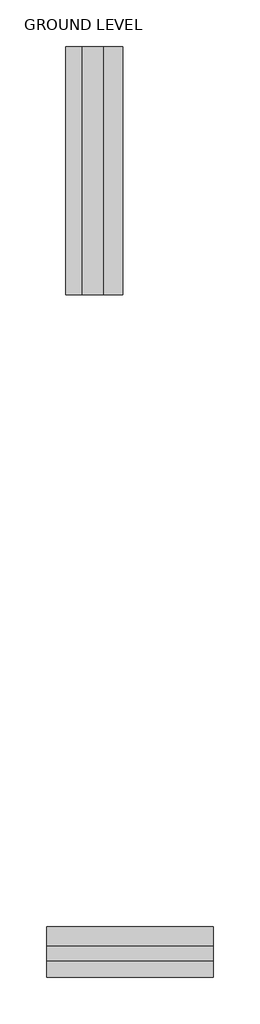
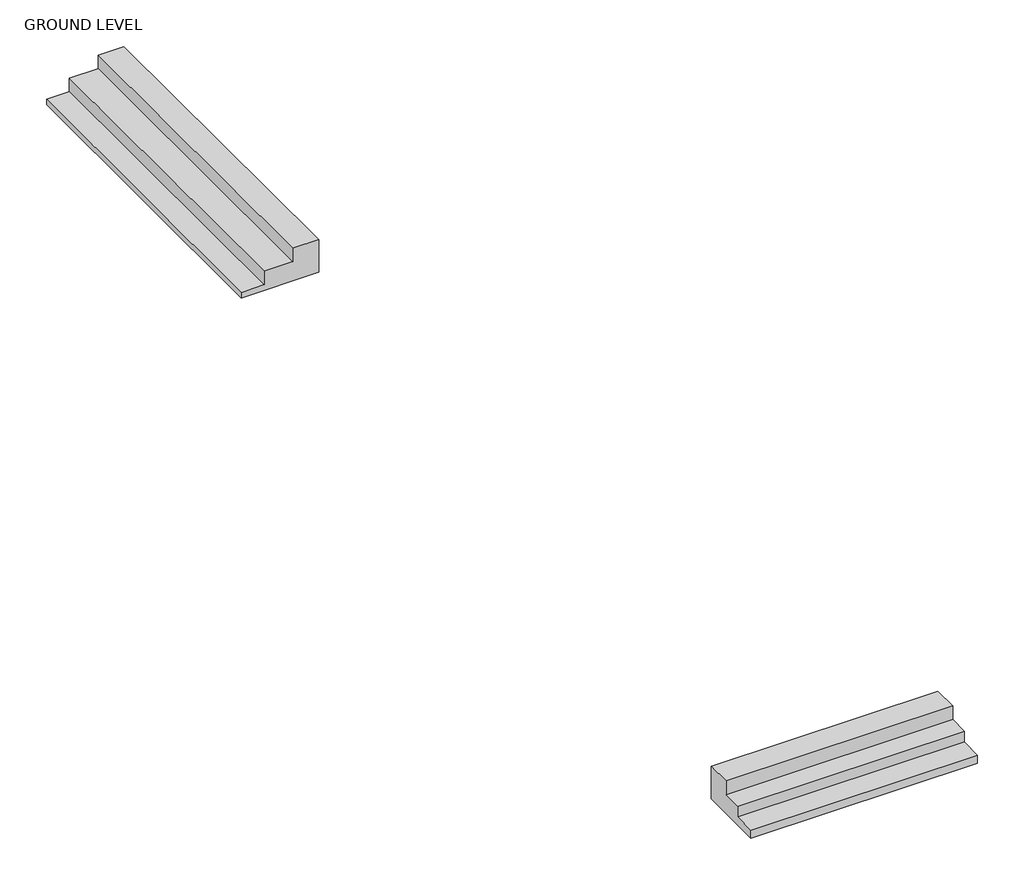
# One storey: 2 proxies.
"""IFC4 building model written with IfcOpenShell, lengths in millimetres."""

from ifc_helpers import new_model, si_unit, origin, place, context, project, spatial, transform, mapped, element, save
from components import generic_models_1_generic_models_1_803bd6b9, generic_models_2_generic_models_2_299d73bb

model = new_model("IFC4")

# Units and contexts
model_context = context("Model", 3, world=origin())
ifc_project = project(units=[si_unit("LENGTHUNIT", "METRE", prefix="MILLI")], contexts=[model_context])

# Site, building, storey
site = spatial("IfcSite", under=ifc_project)
building = spatial("IfcBuilding", under=site)
storey = spatial("IfcBuildingStorey", under=building, Name="GROUND LEVEL", Elevation=0.0)

# Proxies
placement = place(None, origin())
generic_models_1_generic_models_1_shape = generic_models_1_generic_models_1_803bd6b9(model_context)
element("IfcBuildingElementProxy", 1, Name="Generic Models 1 : Generic Models 1", ObjectType="Generic Models 1 : Generic Models 1", at=placement, inside=storey, context=model_context, shape_type="MappedRepresentation", body=[
    mapped(generic_models_1_generic_models_1_shape, transform((0.0, 0.0, 0.0), x_axis=(1.0, 0.0, 0.0), y_axis=(0.0, 1.0, 0.0), z_axis=(0.0, 0.0, 1.0))),
])
generic_models_2_generic_models_2_shape = generic_models_2_generic_models_2_299d73bb(model_context)
element("IfcBuildingElementProxy", 2, Name="Generic Models 2 : Generic Models 2", ObjectType="Generic Models 2 : Generic Models 2", at=placement, inside=storey, context=model_context, shape_type="MappedRepresentation", body=[
    mapped(generic_models_2_generic_models_2_shape, transform((0.0, 0.0, 0.0), x_axis=(1.0, 0.0, 0.0), y_axis=(0.0, 1.0, 0.0), z_axis=(0.0, 0.0, 1.0))),
])

save(model, "model.ifc")

# Revit data of these elements
# Element 1 (IfcBuildingElementProxy, "Generic Models 1 : Generic Models 1")
#   Phase Created = New Construction
#   Materials on its faces: "Clad - White"
# Element 2 (IfcBuildingElementProxy, "Generic Models 2 : Generic Models 2")
#   Phase Created = New Construction
#   Materials on its faces: "Clad - White"
# Materials
#   "Clad - White": class "Wood", colour RGB 242 242 238, transparency 0, Cost = 0
